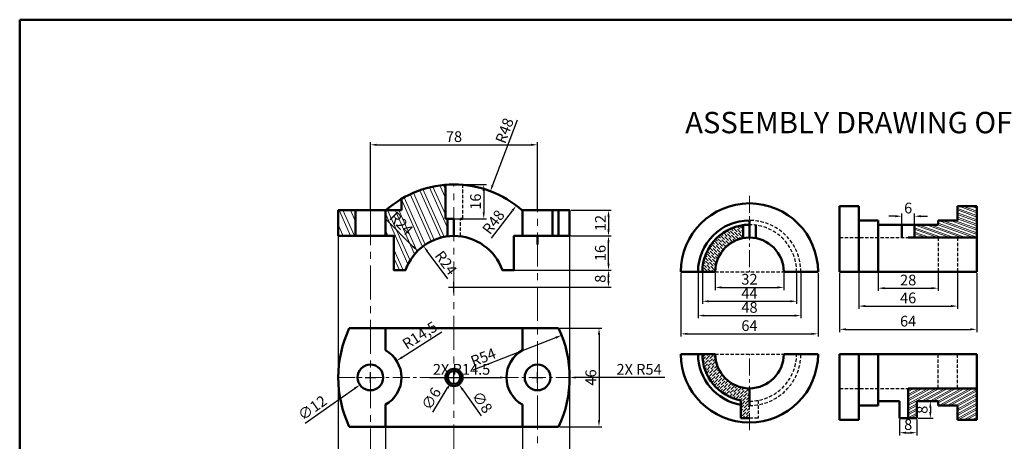
# Model space of a CAD drawing. Units: millimetres. Extents: x 6 to 817, y -61 to 407.
# Tile 2 of 3: x 6 to 466, y 210 to 407. Entities that reach past the tile are written whole.
import ezdxf

# ---------------------------------------------------------------- set-up
doc = ezdxf.new("R2010")
doc.units = ezdxf.units.MM
doc.header["$LTSCALE"] = 0.5
doc.linetypes.add('CENTER', pattern=[50.8, 31.75, -6.35, 6.35, -6.35])
doc.linetypes.add('HIDDEN', pattern=[9.525, 6.35, -3.175])
for name, color, linetype, lineweight in [('M-CNTR', 1, 'CENTER', 18), ('M-DIMS', 2, 'Continuous', 25), ('M-HATC', 8, 'Continuous', 18), ('M-HIDN', 4, 'HIDDEN', 25), ('M-OUTL', 7, 'Continuous', 50), ('M-TEXT', 3, 'Continuous', 25)]:
    doc.layers.add(name, color=color, linetype=linetype, lineweight=lineweight)
doc.styles.get("Standard").update_dxf_attribs({"font": 'arial.ttf'})
doc.dimstyles.new('ISO-25', dxfattribs={"dimtxt": 5, "dimasz": 3, "dimexe": 1.25, "dimexo": 0.625, "dimtad": 1, "dimtxsty": 'Standard', "dimcen": 2.5, "dimadec": 0, "dimazin": 0, "dimtfac": 1, "dimtofl": 0, "dimtmove": 0, "dimatfit": 3, "dimfxl": 1, "dimarcsym": 0})

# ---------------------------------------------------------------- blocks, each defined once
blk = doc.blocks.new('*D19')
at = {"layer": 'Defpoints', "color": 0, "ltscale": 0.5, "transparency": 16777216}
for p in [(257.89, 263.11), (257.89, 217.11), (276.73, 217.11)]:
    blk.add_point(p, dxfattribs=at)
at = {"layer": 'M-DIMS', "color": 0, "lineweight": -2, "ltscale": 0.5, "transparency": 16777216}
for p, q in [((258.51, 263.11), (277.98, 263.11)), ((276.73, 260.11), (276.73, 220.11)), ((258.51, 217.11), (277.98, 217.11))]:
    blk.add_line(p, q, dxfattribs=at)
at = {"layer": 'M-DIMS', "color": 0, "ltscale": 0.5, "transparency": 16777216}
for points in [[(276.23, 260.11), (277.23, 260.11), (276.73, 263.11)], [(276.23, 220.11), (277.23, 220.11), (276.73, 217.11)]]:
    blk.add_solid(points, dxfattribs=at)
at = {"layer": 'M-DIMS', "color": 0, "ltscale": 0.5, "transparency": 16777216, "insert": (273.55, 240.11), "char_height": 5, "attachment_point": 5, "rotation": 90}
blk.add_mtext('46', dxfattribs=at)
blk = doc.blocks.new('*D20')
at = {"layer": 'Defpoints', "color": 0, "ltscale": 0.5, "transparency": 16777216}
for p in [(182.27, 247.89), (170.03, 240.11)]:
    blk.add_point(p, dxfattribs=at)
at = {"layer": 'M-DIMS', "color": 0, "lineweight": -2, "ltscale": 0.5, "transparency": 16777216}
for p, q in [((203.42, 261.33), (184.8, 249.5)), ((167.53, 240.11), (172.53, 240.11)), ((170.03, 237.61), (170.03, 242.61))]:
    blk.add_line(p, q, dxfattribs=at)
at = {"layer": 'M-DIMS', "color": 0, "ltscale": 0.5, "transparency": 16777216}
blk.add_solid([(184.53, 249.92), (185.07, 249.08), (182.27, 247.89)], dxfattribs=at)
at = {"layer": 'M-DIMS', "color": 0, "ltscale": 0.5, "transparency": 16777216, "insert": (193.43, 259.28), "char_height": 5, "attachment_point": 5, "rotation": 32.4428}
blk.add_mtext('R14,5', dxfattribs=at)
blk = doc.blocks.new('*D21')
at = {"layer": 'Defpoints', "color": 0, "ltscale": 0.5, "transparency": 16777216}
for p in [(259.31, 259.81), (209.03, 240.11)]:
    blk.add_point(p, dxfattribs=at)
at = {"layer": 'M-DIMS', "color": 0, "lineweight": -2, "ltscale": 0.5, "transparency": 16777216}
blk.add_line((217.95, 243.6), (256.52, 258.72), dxfattribs=at)
at = {"layer": 'M-DIMS', "color": 0, "ltscale": 0.5, "transparency": 16777216}
blk.add_solid([(256.33, 259.18), (256.7, 258.25), (259.31, 259.81)], dxfattribs=at)
at = {"layer": 'M-DIMS', "color": 0, "ltscale": 0.5, "transparency": 16777216, "insert": (222.93, 248.96), "char_height": 5, "attachment_point": 5, "rotation": 21.398}
blk.add_mtext('R54', dxfattribs=at)
blk = doc.blocks.new('*D22')
at = {"layer": 'Defpoints', "color": 0, "ltscale": 0.5, "transparency": 16777216}
for p in [(174.94, 243.56), (165.12, 236.66)]:
    blk.add_point(p, dxfattribs=at)
at = {"layer": 'M-DIMS', "color": 0, "lineweight": -2, "ltscale": 0.5, "transparency": 16777216}
for p, q in [((167.53, 240.11), (172.53, 240.11)), ((170.03, 237.61), (170.03, 242.61)), ((139.54, 218.71), (162.66, 234.94))]:
    blk.add_line(p, q, dxfattribs=at)
at = {"layer": 'M-DIMS', "color": 0, "ltscale": 0.5, "transparency": 16777216}
blk.add_solid([(162.38, 235.35), (162.95, 234.53), (165.12, 236.66)], dxfattribs=at)
at = {"layer": 'M-DIMS', "color": 0, "ltscale": 0.5, "transparency": 16777216, "insert": (143.29, 225.39), "char_height": 5, "attachment_point": 5, "rotation": 35.0654}
blk.add_mtext('∅12', dxfattribs=at)
blk = doc.blocks.new('*D23')
at = {"layer": 'Defpoints', "color": 0, "ltscale": 0.5, "transparency": 16777216}
for p in [(206.69, 243.36), (211.37, 236.86)]:
    blk.add_point(p, dxfattribs=at)
at = {"layer": 'M-DIMS', "color": 0, "lineweight": -2, "ltscale": 0.5, "transparency": 16777216}
for p, q in [((206.53, 240.11), (211.53, 240.11)), ((209.03, 237.61), (209.03, 242.61)), ((221.92, 222.19), (213.12, 234.43))]:
    blk.add_line(p, q, dxfattribs=at)
at = {"layer": 'M-DIMS', "color": 0, "ltscale": 0.5, "transparency": 16777216}
blk.add_solid([(213.52, 234.72), (212.71, 234.14), (211.37, 236.86)], dxfattribs=at)
at = {"layer": 'M-DIMS', "color": 0, "ltscale": 0.5, "transparency": 16777216, "insert": (221.7, 228.18), "char_height": 5, "attachment_point": 5, "rotation": 305.7354}
blk.add_mtext('∅8', dxfattribs=at)
blk = doc.blocks.new('*D24')
at = {"layer": 'Defpoints', "color": 0, "ltscale": 0.5, "transparency": 16777216}
for p in [(210.58, 242.68), (207.48, 237.54)]:
    blk.add_point(p, dxfattribs=at)
at = {"layer": 'M-DIMS', "color": 0, "lineweight": -2, "ltscale": 0.5, "transparency": 16777216}
for p, q in [((206.53, 240.11), (211.53, 240.11)), ((209.03, 237.61), (209.03, 242.61)), ((199.24, 223.87), (205.93, 234.97))]:
    blk.add_line(p, q, dxfattribs=at)
at = {"layer": 'M-DIMS', "color": 0, "ltscale": 0.5, "transparency": 16777216}
blk.add_solid([(205.51, 235.23), (206.36, 234.71), (207.48, 237.54)], dxfattribs=at)
at = {"layer": 'M-DIMS', "color": 0, "ltscale": 0.5, "transparency": 16777216, "insert": (198.97, 229.85), "char_height": 5, "attachment_point": 5, "rotation": 58.929}
blk.add_mtext('∅6', dxfattribs=at)
blk = doc.blocks.new('*D25')
at = {"layer": 'Defpoints', "color": 0, "ltscale": 0.5, "transparency": 16777216}
for p in [(263.03, 318.23), (263.03, 306.23), (281.16, 306.23)]:
    blk.add_point(p, dxfattribs=at)
at = {"layer": 'M-DIMS', "color": 0, "lineweight": -2, "ltscale": 0.5, "transparency": 16777216}
for p, q in [((263.66, 318.23), (282.41, 318.23)), ((281.16, 315.23), (281.16, 309.23)), ((263.66, 306.23), (282.41, 306.23))]:
    blk.add_line(p, q, dxfattribs=at)
at = {"layer": 'M-DIMS', "color": 0, "ltscale": 0.5, "transparency": 16777216}
for points in [[(280.66, 315.23), (281.66, 315.23), (281.16, 318.23)], [(280.66, 309.23), (281.66, 309.23), (281.16, 306.23)]]:
    blk.add_solid(points, dxfattribs=at)
at = {"layer": 'M-DIMS', "color": 0, "ltscale": 0.5, "transparency": 16777216, "insert": (278.02, 312.23), "char_height": 5, "attachment_point": 5, "rotation": 90}
blk.add_mtext('12', dxfattribs=at)
blk = doc.blocks.new('*D26')
at = {"layer": 'Defpoints', "color": 0, "ltscale": 0.5, "transparency": 16777216}
for p in [(237.03, 306.23), (281.16, 306.23), (237.03, 290.23)]:
    blk.add_point(p, dxfattribs=at)
at = {"layer": 'M-DIMS', "color": 0, "lineweight": -2, "ltscale": 0.5, "transparency": 16777216}
for p, q in [((237.66, 306.23), (282.41, 306.23)), ((281.16, 293.23), (281.16, 303.23)), ((237.66, 290.23), (282.41, 290.23))]:
    blk.add_line(p, q, dxfattribs=at)
at = {"layer": 'M-DIMS', "color": 0, "ltscale": 0.5, "transparency": 16777216}
for points in [[(280.66, 303.23), (281.66, 303.23), (281.16, 306.23)], [(280.66, 293.23), (281.66, 293.23), (281.16, 290.23)]]:
    blk.add_solid(points, dxfattribs=at)
at = {"layer": 'M-DIMS', "color": 0, "ltscale": 0.5, "transparency": 16777216, "insert": (277.98, 298.23), "char_height": 5, "attachment_point": 5, "rotation": 90}
blk.add_mtext('16', dxfattribs=at)
blk = doc.blocks.new('*D27')
at = {"layer": 'Defpoints', "color": 0, "ltscale": 0.5, "transparency": 16777216}
for p in [(231.66, 290.23), (281.16, 290.23), (209.03, 282.23)]:
    blk.add_point(p, dxfattribs=at)
at = {"layer": 'M-DIMS', "color": 0, "lineweight": -2, "ltscale": 0.5, "transparency": 16777216}
for p, q in [((232.28, 290.23), (282.41, 290.23)), ((281.16, 285.23), (281.16, 287.23)), ((209.66, 282.23), (282.41, 282.23))]:
    blk.add_line(p, q, dxfattribs=at)
at = {"layer": 'M-DIMS', "color": 0, "ltscale": 0.5, "transparency": 16777216}
for points in [[(280.66, 287.23), (281.66, 287.23), (281.16, 290.23)], [(280.66, 285.23), (281.66, 285.23), (281.16, 282.23)]]:
    blk.add_solid(points, dxfattribs=at)
at = {"layer": 'M-DIMS', "color": 0, "ltscale": 0.5, "transparency": 16777216, "insert": (277.98, 286.23), "char_height": 5, "attachment_point": 5, "rotation": 90}
blk.add_mtext('8', dxfattribs=at)
blk = doc.blocks.new('*D28')
at = {"layer": 'Defpoints', "color": 0, "ltscale": 0.5, "transparency": 16777216}
for p in [(209.03, 330.23), (209.03, 314.23), (222.93, 314.23)]:
    blk.add_point(p, dxfattribs=at)
at = {"layer": 'M-DIMS', "color": 0, "lineweight": -2, "ltscale": 0.5, "transparency": 16777216}
for p, q in [((209.66, 330.23), (224.18, 330.23)), ((222.93, 327.23), (222.93, 317.23)), ((209.66, 314.23), (224.18, 314.23))]:
    blk.add_line(p, q, dxfattribs=at)
at = {"layer": 'M-DIMS', "color": 0, "ltscale": 0.5, "transparency": 16777216}
for points in [[(222.43, 327.23), (223.43, 327.23), (222.93, 330.23)], [(222.43, 317.23), (223.43, 317.23), (222.93, 314.23)]]:
    blk.add_solid(points, dxfattribs=at)
at = {"layer": 'M-DIMS', "color": 0, "ltscale": 0.5, "transparency": 16777216, "insert": (219.75, 322.23), "char_height": 5, "attachment_point": 5, "rotation": 90}
blk.add_mtext('16', dxfattribs=at)
blk = doc.blocks.new('*D29')
at = {"layer": 'Defpoints', "color": 0, "ltscale": 0.5, "transparency": 16777216}
for p in [(194.8, 301.55), (209.03, 282.23)]:
    blk.add_point(p, dxfattribs=at)
at = {"layer": 'M-DIMS', "color": 0, "lineweight": -2, "ltscale": 0.5, "transparency": 16777216}
blk.add_line((206.17, 286.11), (196.58, 299.14), dxfattribs=at)
at = {"layer": 'M-DIMS', "color": 0, "ltscale": 0.5, "transparency": 16777216}
blk.add_solid([(196.98, 299.43), (196.18, 298.84), (194.8, 301.55)], dxfattribs=at)
at = {"layer": 'M-DIMS', "color": 0, "ltscale": 0.5, "transparency": 16777216, "insert": (204.79, 293.28), "char_height": 5, "attachment_point": 5, "rotation": 306.3657}
blk.add_mtext('R24', dxfattribs=at)
blk = doc.blocks.new('*D30')
at = {"layer": 'Defpoints', "color": 0, "ltscale": 0.5, "transparency": 16777216}
for p in [(238.13, 320.4), (209.03, 282.23)]:
    blk.add_point(p, dxfattribs=at)
at = {"layer": 'M-DIMS', "color": 0, "lineweight": -2, "ltscale": 0.5, "transparency": 16777216}
blk.add_line((226.48, 305.13), (236.31, 318.02), dxfattribs=at)
at = {"layer": 'M-DIMS', "color": 0, "ltscale": 0.5, "transparency": 16777216}
blk.add_solid([(235.91, 318.32), (236.71, 317.71), (238.13, 320.4)], dxfattribs=at)
at = {"layer": 'M-DIMS', "color": 0, "ltscale": 0.5, "transparency": 16777216, "insert": (227.96, 312.31), "char_height": 5, "attachment_point": 5, "rotation": 52.6886}
blk.add_mtext('R48', dxfattribs=at)
blk = doc.blocks.new('*D31')
at = {"layer": 'Defpoints', "color": 0, "ltscale": 0.5, "transparency": 16777216}
for p in [(330.95, 289.45), (362.95, 289.45), (362.95, 282.17)]:
    blk.add_point(p, dxfattribs=at)
at = {"layer": 'M-DIMS', "color": 0, "lineweight": -2, "ltscale": 0.5, "transparency": 16777216}
for p, q in [((330.95, 288.83), (330.95, 280.92)), ((362.95, 288.83), (362.95, 280.92)), ((333.95, 282.17), (359.95, 282.17))]:
    blk.add_line(p, q, dxfattribs=at)
at = {"layer": 'M-DIMS', "color": 0, "ltscale": 0.5, "transparency": 16777216}
for points in [[(333.95, 282.67), (333.95, 281.67), (330.95, 282.17)], [(359.95, 282.67), (359.95, 281.67), (362.95, 282.17)]]:
    blk.add_solid(points, dxfattribs=at)
at = {"layer": 'M-DIMS', "color": 0, "ltscale": 0.5, "transparency": 16777216, "insert": (346.95, 285.35), "char_height": 5, "attachment_point": 5}
blk.add_mtext('32', dxfattribs=at)
blk = doc.blocks.new('*D32')
at = {"layer": 'Defpoints', "color": 0, "ltscale": 0.5, "transparency": 16777216}
for p in [(324.95, 289.45), (368.95, 289.45), (368.95, 275.69)]:
    blk.add_point(p, dxfattribs=at)
at = {"layer": 'M-DIMS', "color": 0, "lineweight": -2, "ltscale": 0.5, "transparency": 16777216}
for p, q in [((324.95, 288.83), (324.95, 274.44)), ((368.95, 288.83), (368.95, 274.44)), ((327.95, 275.69), (365.95, 275.69))]:
    blk.add_line(p, q, dxfattribs=at)
at = {"layer": 'M-DIMS', "color": 0, "ltscale": 0.5, "transparency": 16777216}
for points in [[(327.95, 276.19), (327.95, 275.19), (324.95, 275.69)], [(365.95, 276.19), (365.95, 275.19), (368.95, 275.69)]]:
    blk.add_solid(points, dxfattribs=at)
at = {"layer": 'M-DIMS', "color": 0, "ltscale": 0.5, "transparency": 16777216, "insert": (346.95, 278.81), "char_height": 5, "attachment_point": 5}
blk.add_mtext('44', dxfattribs=at)
blk = doc.blocks.new('*D33')
at = {"layer": 'Defpoints', "color": 0, "ltscale": 0.5, "transparency": 16777216}
for p in [(322.95, 289.45), (370.95, 289.45), (370.95, 269.02)]:
    blk.add_point(p, dxfattribs=at)
at = {"layer": 'M-DIMS', "color": 0, "lineweight": -2, "ltscale": 0.5, "transparency": 16777216}
for p, q in [((322.95, 288.83), (322.95, 267.77)), ((370.95, 288.83), (370.95, 267.77)), ((325.95, 269.02), (367.95, 269.02))]:
    blk.add_line(p, q, dxfattribs=at)
at = {"layer": 'M-DIMS', "color": 0, "ltscale": 0.5, "transparency": 16777216}
for points in [[(325.95, 269.52), (325.95, 268.52), (322.95, 269.02)], [(367.95, 269.52), (367.95, 268.52), (370.95, 269.02)]]:
    blk.add_solid(points, dxfattribs=at)
at = {"layer": 'M-DIMS', "color": 0, "ltscale": 0.5, "transparency": 16777216, "insert": (346.95, 272.19), "char_height": 5, "attachment_point": 5}
blk.add_mtext('48', dxfattribs=at)
blk = doc.blocks.new('*D34')
at = {"layer": 'Defpoints', "color": 0, "ltscale": 0.5, "transparency": 16777216}
for p in [(314.95, 289.45), (378.95, 289.45), (378.95, 260.49)]:
    blk.add_point(p, dxfattribs=at)
at = {"layer": 'M-DIMS', "color": 0, "lineweight": -2, "ltscale": 0.5, "transparency": 16777216}
for p, q in [((314.95, 288.83), (314.95, 259.24)), ((378.95, 288.83), (378.95, 259.24)), ((317.95, 260.49), (375.95, 260.49))]:
    blk.add_line(p, q, dxfattribs=at)
at = {"layer": 'M-DIMS', "color": 0, "ltscale": 0.5, "transparency": 16777216}
for points in [[(317.95, 260.99), (317.95, 259.99), (314.95, 260.49)], [(375.95, 260.99), (375.95, 259.99), (378.95, 260.49)]]:
    blk.add_solid(points, dxfattribs=at)
at = {"layer": 'M-DIMS', "color": 0, "ltscale": 0.5, "transparency": 16777216, "insert": (346.95, 263.67), "char_height": 5, "attachment_point": 5}
blk.add_mtext('64', dxfattribs=at)
blk = doc.blocks.new('*D35')
at = {"layer": 'Defpoints', "color": 0, "ltscale": 0.5, "transparency": 16777216}
for p in [(417.01, 221.03), (425.01, 221.03), (425.01, 214.3)]:
    blk.add_point(p, dxfattribs=at)
at = {"layer": 'M-DIMS', "color": 0, "lineweight": -2, "ltscale": 0.5, "transparency": 16777216}
for p, q in [((417.01, 220.41), (417.01, 213.05)), ((425.01, 220.41), (425.01, 213.05)), ((420.01, 214.3), (422.01, 214.3))]:
    blk.add_line(p, q, dxfattribs=at)
at = {"layer": 'M-DIMS', "color": 0, "ltscale": 0.5, "transparency": 16777216}
for points in [[(420.01, 214.8), (420.01, 213.8), (417.01, 214.3)], [(422.01, 214.8), (422.01, 213.8), (425.01, 214.3)]]:
    blk.add_solid(points, dxfattribs=at)
at = {"layer": 'M-DIMS', "color": 0, "ltscale": 0.5, "transparency": 16777216, "insert": (421.01, 217.48), "char_height": 5, "attachment_point": 5}
blk.add_mtext('8', dxfattribs=at)
blk = doc.blocks.new('*D36')
at = {"layer": 'Defpoints', "color": 0, "ltscale": 0.5, "transparency": 16777216}
for p in [(425.03, 229.03), (425.03, 221.03), (431.36, 221.03)]:
    blk.add_point(p, dxfattribs=at)
at = {"layer": 'M-DIMS', "color": 0, "lineweight": -2, "ltscale": 0.5, "transparency": 16777216}
for p, q in [((425.65, 229.03), (432.61, 229.03)), ((431.36, 226.03), (431.36, 224.03)), ((425.65, 221.03), (432.61, 221.03))]:
    blk.add_line(p, q, dxfattribs=at)
at = {"layer": 'M-DIMS', "color": 0, "ltscale": 0.5, "transparency": 16777216}
for points in [[(430.86, 226.03), (431.86, 226.03), (431.36, 229.03)], [(430.86, 224.03), (431.86, 224.03), (431.36, 221.03)]]:
    blk.add_solid(points, dxfattribs=at)
at = {"layer": 'M-DIMS', "color": 0, "ltscale": 0.5, "transparency": 16777216, "insert": (428.18, 225.03), "char_height": 5, "attachment_point": 5, "rotation": 90}
blk.add_mtext('8', dxfattribs=at)
blk = doc.blocks.new('*D37')
at = {"layer": 'Defpoints', "color": 0, "ltscale": 0.5, "transparency": 16777216}
for p in [(407.01, 289.45), (435.01, 289.45), (435.01, 281.8)]:
    blk.add_point(p, dxfattribs=at)
at = {"layer": 'M-DIMS', "color": 0, "lineweight": -2, "ltscale": 0.5, "transparency": 16777216}
for p, q in [((407.01, 288.83), (407.01, 280.55)), ((435.01, 288.83), (435.01, 280.55)), ((410.01, 281.8), (432.01, 281.8))]:
    blk.add_line(p, q, dxfattribs=at)
at = {"layer": 'M-DIMS', "color": 0, "ltscale": 0.5, "transparency": 16777216}
for points in [[(410.01, 282.3), (410.01, 281.3), (407.01, 281.8)], [(432.01, 282.3), (432.01, 281.3), (435.01, 281.8)]]:
    blk.add_solid(points, dxfattribs=at)
at = {"layer": 'M-DIMS', "color": 0, "ltscale": 0.5, "transparency": 16777216, "insert": (421.01, 284.98), "char_height": 5, "attachment_point": 5}
blk.add_mtext('28', dxfattribs=at)
blk = doc.blocks.new('*D38')
at = {"layer": 'Defpoints', "color": 0, "ltscale": 0.5, "transparency": 16777216}
for p in [(398.01, 289.45), (444.01, 289.45), (444.01, 273.46)]:
    blk.add_point(p, dxfattribs=at)
at = {"layer": 'M-DIMS', "color": 0, "lineweight": -2, "ltscale": 0.5, "transparency": 16777216}
for p, q in [((398.01, 288.83), (398.01, 272.21)), ((444.01, 288.83), (444.01, 272.21)), ((401.01, 273.46), (441.01, 273.46))]:
    blk.add_line(p, q, dxfattribs=at)
at = {"layer": 'M-DIMS', "color": 0, "ltscale": 0.5, "transparency": 16777216}
for points in [[(401.01, 273.96), (401.01, 272.96), (398.01, 273.46)], [(441.01, 273.96), (441.01, 272.96), (444.01, 273.46)]]:
    blk.add_solid(points, dxfattribs=at)
at = {"layer": 'M-DIMS', "color": 0, "ltscale": 0.5, "transparency": 16777216, "insert": (421.01, 276.64), "char_height": 5, "attachment_point": 5}
blk.add_mtext('46', dxfattribs=at)
blk = doc.blocks.new('*D39')
at = {"layer": 'Defpoints', "color": 0, "ltscale": 0.5, "transparency": 16777216}
for p in [(389.01, 289.45), (453.01, 289.45), (453.01, 262.59)]:
    blk.add_point(p, dxfattribs=at)
at = {"layer": 'M-DIMS', "color": 0, "lineweight": -2, "ltscale": 0.5, "transparency": 16777216}
for p, q in [((389.01, 288.83), (389.01, 261.34)), ((453.01, 288.83), (453.01, 261.34)), ((392.01, 262.59), (450.01, 262.59))]:
    blk.add_line(p, q, dxfattribs=at)
at = {"layer": 'M-DIMS', "color": 0, "ltscale": 0.5, "transparency": 16777216}
for points in [[(392.01, 263.09), (392.01, 262.09), (389.01, 262.59)], [(450.01, 263.09), (450.01, 262.09), (453.01, 262.59)]]:
    blk.add_solid(points, dxfattribs=at)
at = {"layer": 'M-DIMS', "color": 0, "ltscale": 0.5, "transparency": 16777216, "insert": (421.01, 265.77), "char_height": 5, "attachment_point": 5}
blk.add_mtext('64', dxfattribs=at)
blk = doc.blocks.new('*D40')
at = {"layer": 'Defpoints', "color": 0, "ltscale": 0.5, "transparency": 16777216}
for p in [(424.01, 315.42), (418.01, 311.45), (424.01, 311.45)]:
    blk.add_point(p, dxfattribs=at)
at = {"layer": 'M-DIMS', "color": 0, "lineweight": -2, "ltscale": 0.5, "transparency": 16777216}
for p, q in [((415.01, 315.42), (412.01, 315.42)), ((418.01, 312.08), (418.01, 316.67)), ((424.01, 312.08), (424.01, 316.67)), ((427.01, 315.42), (430.01, 315.42))]:
    blk.add_line(p, q, dxfattribs=at)
at = {"layer": 'M-DIMS', "color": 0, "ltscale": 0.5, "transparency": 16777216}
for points in [[(415.01, 315.92), (415.01, 314.92), (418.01, 315.42)], [(427.01, 315.92), (427.01, 314.92), (424.01, 315.42)]]:
    blk.add_solid(points, dxfattribs=at)
at = {"layer": 'M-DIMS', "color": 0, "ltscale": 0.5, "transparency": 16777216, "insert": (421.01, 318.6), "char_height": 5, "attachment_point": 5}
blk.add_mtext('6', dxfattribs=at)
blk = doc.blocks.new('*D51')
at = {"layer": 'Defpoints', "color": 0, "ltscale": 0.5, "transparency": 16777216}
for p in [(155.03, 306.23), (263.03, 306.23), (263.03, 5.88)]:
    blk.add_point(p, dxfattribs=at)
at = {"layer": 'M-DIMS', "color": 0, "lineweight": -2, "ltscale": 0.5, "transparency": 16777216}
for p, q in [((155.03, 305.6), (155.03, 4.63)), ((263.03, 305.6), (263.03, 4.63)), ((158.03, 5.88), (260.03, 5.88))]:
    blk.add_line(p, q, dxfattribs=at)
at = {"layer": 'M-DIMS', "color": 0, "ltscale": 0.5, "transparency": 16777216}
for points in [[(158.03, 6.38), (158.03, 5.38), (155.03, 5.88)], [(260.03, 6.38), (260.03, 5.38), (263.03, 5.88)]]:
    blk.add_solid(points, dxfattribs=at)
at = {"layer": 'M-DIMS', "color": 0, "ltscale": 0.5, "transparency": 16777216, "insert": (209.03, 9.06), "char_height": 5, "attachment_point": 5}
blk.add_mtext('108', dxfattribs=at)
blk = doc.blocks.new('*D52')
at = {"layer": 'Defpoints', "color": 0, "ltscale": 0.5, "transparency": 16777216}
for p in [(248.03, 348.78), (170.03, 318.23), (248.03, 318.23)]:
    blk.add_point(p, dxfattribs=at)
at = {"layer": 'M-DIMS', "color": 0, "lineweight": -2, "ltscale": 0.5, "transparency": 16777216}
for p, q in [((170.03, 318.85), (170.03, 350.03)), ((248.03, 318.85), (248.03, 350.03)), ((173.03, 348.78), (245.03, 348.78))]:
    blk.add_line(p, q, dxfattribs=at)
at = {"layer": 'M-DIMS', "color": 0, "ltscale": 0.5, "transparency": 16777216}
for points in [[(173.03, 349.28), (173.03, 348.28), (170.03, 348.78)], [(245.03, 349.28), (245.03, 348.28), (248.03, 348.78)]]:
    blk.add_solid(points, dxfattribs=at)
at = {"layer": 'M-DIMS', "color": 0, "ltscale": 0.5, "transparency": 16777216, "insert": (209.03, 351.96), "char_height": 5, "attachment_point": 5}
blk.add_mtext('78', dxfattribs=at)
blk = doc.blocks.new('*D53')
at = {"layer": 'Defpoints', "color": 0, "ltscale": 0.5, "transparency": 16777216}
for p in [(177.03, 217.11), (241.03, 217.11), (241.03, 5.88)]:
    blk.add_point(p, dxfattribs=at)
at = {"layer": 'M-DIMS', "color": 0, "lineweight": -2, "ltscale": 0.5, "transparency": 16777216}
for p, q in [((177.03, 216.48), (177.03, 4.63)), ((241.03, 216.48), (241.03, 4.63)), ((180.03, 5.88), (238.03, 5.88))]:
    blk.add_line(p, q, dxfattribs=at)
at = {"layer": 'M-DIMS', "color": 0, "ltscale": 0.5, "transparency": 16777216}
for points in [[(180.03, 6.38), (180.03, 5.38), (177.03, 5.88)], [(238.03, 6.38), (238.03, 5.38), (241.03, 5.88)]]:
    blk.add_solid(points, dxfattribs=at)
at = {"layer": 'M-DIMS', "color": 0, "ltscale": 0.5, "transparency": 16777216, "insert": (209.03, 9.06), "char_height": 5, "attachment_point": 5}
blk.add_mtext('64', dxfattribs=at)
blk = doc.blocks.new('*D57')
at = {"layer": 'Defpoints', "color": 0, "ltscale": 0.5, "transparency": 16777216}
for p in [(226.01, 327.12), (209.03, 282.23)]:
    blk.add_point(p, dxfattribs=at)
at = {"layer": 'M-DIMS', "color": 0, "lineweight": -2, "ltscale": 0.5, "transparency": 16777216}
for p, q in [((238.53, 360.24), (227.07, 329.93)), ((206.53, 282.23), (211.53, 282.23)), ((209.03, 279.73), (209.03, 284.73))]:
    blk.add_line(p, q, dxfattribs=at)
at = {"layer": 'M-DIMS', "color": 0, "ltscale": 0.5, "transparency": 16777216}
blk.add_solid([(226.6, 330.11), (227.54, 329.75), (226.01, 327.12)], dxfattribs=at)
at = {"layer": 'M-DIMS', "color": 0, "ltscale": 0.5, "transparency": 16777216, "insert": (233.22, 355.19), "char_height": 5, "attachment_point": 5, "rotation": 69.2852}
blk.add_mtext('R48', dxfattribs=at)
blk = doc.blocks.new('*D58')
at = {"layer": 'Defpoints', "color": 0, "ltscale": 0.5, "transparency": 16777216}
for p in [(192.03, 299.17), (209.03, 282.23)]:
    blk.add_point(p, dxfattribs=at)
at = {"layer": 'M-DIMS', "color": 0, "lineweight": -2, "ltscale": 0.5, "transparency": 16777216}
for p, q in [((177.16, 313.98), (189.91, 301.29)), ((206.53, 282.23), (211.53, 282.23)), ((209.03, 279.73), (209.03, 284.73))]:
    blk.add_line(p, q, dxfattribs=at)
at = {"layer": 'M-DIMS', "color": 0, "ltscale": 0.5, "transparency": 16777216}
blk.add_solid([(190.26, 301.64), (189.55, 300.93), (192.03, 299.17)], dxfattribs=at)
at = {"layer": 'M-DIMS', "color": 0, "ltscale": 0.5, "transparency": 16777216, "insert": (184.04, 311.55), "char_height": 5, "attachment_point": 5, "rotation": 315.0976}
blk.add_mtext('R24', dxfattribs=at)
blk = doc.blocks.new('*D59')
at = {"layer": 'Defpoints', "color": 0, "ltscale": 0.5, "transparency": 16777216}
for p in [(233.53, 240.1), (248.03, 240.11)]:
    blk.add_point(p, dxfattribs=at)
at = {"layer": 'M-DIMS', "color": 0, "lineweight": -2, "ltscale": 0.5, "transparency": 16777216}
for p, q in [((197.64, 240.08), (230.53, 240.1)), ((245.53, 240.11), (250.53, 240.11)), ((248.03, 237.61), (248.03, 242.61))]:
    blk.add_line(p, q, dxfattribs=at)
at = {"layer": 'M-DIMS', "color": 0, "ltscale": 0.5, "transparency": 16777216}
blk.add_solid([(230.53, 240.6), (230.53, 239.6), (233.53, 240.1)], dxfattribs=at)
at = {"layer": 'M-DIMS', "color": 0, "ltscale": 0.5, "transparency": 16777216, "insert": (212.58, 243.26), "char_height": 5, "attachment_point": 5, "rotation": 0.0366}
blk.add_mtext('2X R14.5', dxfattribs=at)
blk = doc.blocks.new('*D60')
at = {"layer": 'Defpoints', "color": 0, "ltscale": 0.5, "transparency": 16777216}
for p in [(209.03, 240.11), (263.03, 240.1)]:
    blk.add_point(p, dxfattribs=at)
at = {"layer": 'M-DIMS', "color": 0, "lineweight": -2, "ltscale": 0.5, "transparency": 16777216}
for p, q in [((206.53, 240.11), (211.53, 240.11)), ((209.03, 237.61), (209.03, 242.61)), ((307.43, 240.09), (266.03, 240.1))]:
    blk.add_line(p, q, dxfattribs=at)
at = {"layer": 'M-DIMS', "color": 0, "ltscale": 0.5, "transparency": 16777216}
blk.add_solid([(266.03, 240.6), (266.03, 239.6), (263.03, 240.1)], dxfattribs=at)
at = {"layer": 'M-DIMS', "color": 0, "ltscale": 0.5, "transparency": 16777216, "insert": (295.43, 243.27), "char_height": 5, "attachment_point": 5, "rotation": 359.9901}
blk.add_mtext('2X R54', dxfattribs=at)

msp = doc.modelspace()

# ---------------------------------------------------------------- hatches: boundary and pattern name
at = {"layer": 'M-HATC', "ltscale": 0.5}
h = msp.add_hatch(dxfattribs=at)
h.set_pattern_fill('ANSI32', color=256, scale=0.5, angle=69)
h.paths.add_polyline_path([(206.031, 314.227), (205.031, 314.227), (205.031, 330.06, 0.113544), (184.531, 323.504), (184.531, 318.227), (177.282, 318.227), (177.031, 318.227), (177.031, 306.227), (181.031, 306.227), (181.031, 302.227), (181.031, 290.227), (186.403, 290.227, -0.2836692), (206.031, 306.039)])
h.paths.add_polyline_path([(163.031, 318.227), (155.031, 318.227), (155.031, 306.227), (163.031, 306.227)])
h = msp.add_hatch(dxfattribs=at)
h.set_pattern_fill('ANSI32', color=256, scale=0.2, angle=115)
h.set_pattern_definition([(160, (-84.5117, -12.3327), (-0.6515484, -1.7901144), []), (160, (-84.8912, -11.5188), (-0.6515484, -1.7901144), [])])
h.paths.add_polyline_path([(453.012, 305.451), (453.012, 320.152), (444.012, 320.152), (444.012, 313.451), (435.012, 313.451), (435.012, 311.451), (424.012, 311.451), (424.012, 305.451)])
h = msp.add_hatch(dxfattribs=at)
h.set_pattern_fill('ANSI36', color=256, scale=0.3, angle=90)
h.paths.add_polyline_path([(343.952, 311.246, 0.3746932), (324.952, 289.451), (330.952, 289.451, -0.359988), (343.952, 305.168)])
h = msp.add_hatch(dxfattribs=at)
h.set_pattern_fill('ANSI36', color=256, scale=0.3)
h.paths.add_polyline_path([(330.952, 251.033), (324.952, 251.033, 0.3616215), (342.952, 229.4), (342.952, 221.033), (346.952, 221.033), (346.952, 235.033, -0.4142136)])
h = msp.add_hatch(dxfattribs=at)
h.set_pattern_fill('ANSI32', color=256, scale=0.2, angle=164)
h.set_pattern_definition([(209, (-84.5117, -22.6975), (0.9235623, -1.6661505), []), (209, (-85.375, -22.45), (0.9235623, -1.6661505), [])])
h.paths.add_polyline_path([(444.012, 227.033), (444.012, 220.332), (453.012, 220.332), (453.012, 235.033), (421.012, 235.033), (421.012, 221.033), (425.012, 221.033), (425.012, 229.033), (435.012, 229.033), (435.012, 227.033)])

# ---------------------------------------------------------------- linework, layer by layer
at = {"layer": 'M-CNTR'}
for p, q in [((209.031, 24.431), (209.031, 330.227)), ((170.031, 124.143), (170.031, 318.227)), ((248.031, 114.143), (248.031, 318.227))]:
    msp.add_line(p, q, dxfattribs=at)
at = {"layer": 'M-CNTR', "ltscale": 0.5}
for p, q in [((346.952, 324.926), (346.952, 289.451)), ((346.952, 215.559), (346.952, 251.033)), ((155.031, 240.109), (263.031, 240.109))]:
    msp.add_line(p, q, dxfattribs=at)
at = {"layer": 'M-HIDN', "ltscale": 0.5}
for p, q in [((213.031, 330.227), (213.031, 314.227)), ((209.031, 314.227), (212.031, 314.227)), ((212.031, 306.227), (212.031, 314.227)), ((389.012, 305.451), (421.012, 305.451)), ((435.012, 305.451), (435.012, 289.451)), ((444.012, 305.451), (444.012, 289.451)), ((330.952, 289.451), (362.952, 289.451)), ((330.952, 251.033), (362.952, 251.033)), ((435.012, 235.033), (435.012, 251.033)), ((444.012, 235.033), (444.012, 251.033)), ((389.012, 235.033), (421.012, 235.033)), ((350.952, 229.4), (350.952, 221.033)), ((350.952, 221.033), (346.952, 221.033))]:
    msp.add_line(p, q, dxfattribs=at)
for centre, radius, start, end in [((346.952, 289.451), 24, 0, 90), ((346.952, 289.451), 22, 0, 90), ((346.952, 251.033), 22, 270, 0), ((346.952, 251.033), 24, 270, 0)]:
    msp.add_arc(centre, radius, start, end, dxfattribs=at)
at = {"layer": 'M-OUTL', "ltscale": 0.5}
for p, q in [((205.031, 330.227), (205.031, 314.227)), ((184.531, 318.227), (184.531, 323.504)), ((163.031, 318.227), (163.031, 306.227)), ((177.031, 318.227), (177.031, 306.227)), ((177.282, 318.227), (184.531, 318.227)), ((241.031, 306.227), (241.031, 318.227)), ((255.031, 306.227), (255.031, 318.227)), ((257.888, 306.227), (257.888, 318.227)), ((263.031, 306.227), (263.031, 318.227)), ((389.012, 320.152), (389.012, 289.451)), ((389.012, 320.152), (398.012, 320.152)), ((398.012, 320.152), (398.012, 289.451)), ((444.012, 320.152), (444.012, 313.451)), ((444.012, 320.152), (453.012, 320.152)), ((453.012, 320.152), (453.012, 289.451)), ((205.031, 314.227), (209.031, 314.227)), ((206.031, 306.039), (206.031, 314.227)), ((209.031, 306.227), (209.031, 314.227)), ((212.031, 314.227), (213.031, 314.227)), ((346.952, 311.451), (346.952, 313.451)), ((346.952, 313.451), (346.952, 305.451)), ((398.012, 313.451), (407.012, 313.451)), ((407.012, 313.451), (407.012, 289.451)), ((435.012, 313.451), (435.012, 311.451)), ((435.012, 313.451), (444.012, 313.451)), ((343.952, 311.246), (343.952, 305.168)), ((349.952, 311.246), (349.952, 305.168)), ((407.012, 311.451), (435.012, 311.451)), ((418.012, 311.451), (418.012, 305.451)), ((424.012, 311.451), (424.012, 305.451)), ((248.031, 302.227), (248.031, 306.227)), ((421.012, 305.451), (453.012, 305.451)), ((314.952, 289.451), (330.952, 289.451)), ((362.952, 289.451), (378.952, 289.451)), ((389.012, 289.451), (453.012, 289.451)), ((160.174, 263.109), (257.888, 263.109)), ((177.031, 252.808), (177.031, 263.109)), ((241.031, 252.808), (241.031, 263.109)), ((314.952, 251.033), (330.952, 251.033)), ((362.952, 251.033), (378.952, 251.033)), ((389.012, 220.332), (389.012, 251.033)), ((389.012, 251.033), (453.012, 251.033)), ((398.012, 220.332), (398.012, 251.033)), ((407.012, 227.033), (407.012, 251.033)), ((453.012, 220.332), (453.012, 251.033)), ((346.952, 227.033), (346.952, 235.033)), ((421.012, 235.033), (453.012, 235.033)), ((421.012, 221.033), (421.012, 235.033)), ((177.031, 217.109), (177.031, 227.411)), ((241.031, 217.109), (241.031, 227.411)), ((342.952, 229.4), (342.952, 221.033)), ((398.012, 227.033), (407.012, 227.033)), ((407.012, 229.033), (417.012, 229.033)), ((417.012, 221.033), (417.012, 229.033)), ((425.012, 229.033), (425.012, 221.033)), ((425.012, 229.033), (435.012, 229.033)), ((435.012, 227.033), (435.012, 229.033)), ((435.012, 227.033), (444.012, 227.033)), ((444.012, 220.332), (444.012, 227.033)), ((346.952, 221.033), (342.952, 221.033)), ((425.012, 221.033), (417.012, 221.033)), ((160.174, 217.109), (257.888, 217.109)), ((389.012, 220.332), (398.012, 220.332)), ((444.012, 220.332), (453.012, 220.332))]:
    msp.add_line(p, q, dxfattribs=at)
msp.add_lwpolyline([(6.354, 407.228), (817.271, 407.228), (817.271, -60.955), (6.354, -60.955)], close=True, dxfattribs=at)
for points in [[(209.031, 330.227, 0.1826758), (177.282, 318.227), (155.031, 318.227), (155.031, 306.227), (181.031, 306.227), (181.031, 302.227), (181.031, 290.227), (186.403, 290.227, -0.3178372), (209.031, 306.227)], [(209.031, 330.227, -0.1826758), (240.78, 318.227), (263.031, 318.227), (263.031, 306.227), (237.031, 306.227), (237.031, 302.227), (237.031, 290.227), (231.658, 290.227, 0.3178372), (209.031, 306.227)]]:
    msp.add_lwpolyline(points, format="xyb", dxfattribs=at)
for centre, radius in [((170.031, 240.109), 6), ((209.031, 240.109), 4), ((248.031, 240.109), 6), ((209.031, 240.109), 3)]:
    msp.add_circle(centre, radius, dxfattribs=at)
for centre, radius, start, end in [((346.952, 289.451), 32, 0, 180), ((346.952, 289.451), 24, 90, 180), ((346.952, 289.451), 22, 90, 180), ((346.952, 289.451), 16, 0, 180), ((209.031, 240.109), 54, 154.79071, 205.20929), ((209.031, 240.109), 54, 334.79071, 25.20929), ((170.031, 240.109), 14.5, 298.86573, 61.13427), ((248.031, 240.109), 14.5, 118.86573, 241.13427), ((346.952, 251.033), 32, 180, 0), ((346.952, 251.033), 24, 180, 260.40593), ((346.952, 251.033), 22, 180, 259.52432), ((346.952, 251.033), 16, 180, 0)]:
    msp.add_arc(centre, radius, start, end, dxfattribs=at)

# ---------------------------------------------------------------- texts
at = {"layer": 'M-TEXT', "ltscale": 0.5, "insert": (316.953, 364.17), "char_height": 10, "attachment_point": 1}
msp.add_mtext_dynamic_manual_height_columns('ASSEMBLY DRAWING OF PLUMMER BLOCK', width=345.85464, gutter_width=12.5, heights=[0], dxfattribs=at)

# ---------------------------------------------------------------- dimensions: what is measured, and where the dimension line sits
at = {"layer": 'M-DIMS', "ltscale": 0.5}
for center, mpoint, override, picture, middle in [((209.031, 282.227), (226.009, 327.124), {"dimdec": 0, "dimlfac": 1, "dimrnd": 0, "dimzin": 0, "dimdsep": 46, "dimlunit": 2}, '*D57', (236.196, 354.062)), ((209.031, 282.227), (192.031, 299.169), {"dimdec": 0, "dimlfac": 1, "dimrnd": 0, "dimzin": 0, "dimdsep": 46, "dimlunit": 2}, '*D58', (181.832, 309.334)), ((209.031, 282.227), (238.126, 320.404), {"dimclrd": 0, "dimclre": 0, "dimclrt": 0}, '*D30', (230.486, 310.38)), ((209.031, 282.227), (194.8, 301.553), {"dimclrd": 0, "dimclre": 0, "dimclrt": 0}, '*D29', (202.264, 291.416)), ((209.031, 240.109), (259.308, 259.811), {"dimclrd": 0, "dimclre": 0, "dimclrt": 0}, '*D21', (224.083, 246.007))]:
    dim = msp.add_radius_dim(center=center, mpoint=mpoint, dimstyle='ISO-25', override=override, dxfattribs=at)
    dim.commit()
    dim.dimension.update_dxf_attribs({"geometry": picture, "text_midpoint": middle, "dimtype": 164})
for base, p1, p2, override, picture, middle in [((248.031, 348.777), (170.031, 318.227), (248.031, 318.227), {"dimdec": 0, "dimlfac": 1, "dimrnd": 0, "dimzin": 0, "dimdsep": 46, "dimlunit": 2}, '*D52', (209.031, 351.955)), ((424.012, 315.42), (418.012, 311.451), (424.012, 311.451), {"dimclrd": 0, "dimclre": 0, "dimclrt": 0}, '*D40', (421.012, 318.598)), ((263.031, 5.881), (155.031, 306.227), (263.031, 306.227), {"dimdec": 0, "dimlfac": 1, "dimrnd": 0, "dimzin": 0, "dimdsep": 46, "dimlunit": 2}, '*D51', (209.031, 9.059)), ((378.952, 260.489), (314.952, 289.451), (378.952, 289.451), {"dimclrd": 0, "dimclre": 0, "dimclrt": 0}, '*D34', (346.952, 263.666)), ((370.952, 269.016), (322.952, 289.451), (370.952, 289.451), {"dimclrd": 0, "dimclre": 0, "dimclrt": 0}, '*D33', (346.952, 272.194)), ((368.952, 275.689), (324.952, 289.451), (368.952, 289.451), {"dimclrd": 0, "dimclre": 0, "dimclrt": 0}, '*D32', (346.952, 278.814)), ((362.952, 282.169), (330.952, 289.451), (362.952, 289.451), {"dimclrd": 0, "dimclre": 0, "dimclrt": 0}, '*D31', (346.952, 285.349)), ((453.012, 262.591), (389.012, 289.451), (453.012, 289.451), {"dimclrd": 0, "dimclre": 0, "dimclrt": 0}, '*D39', (421.012, 265.769)), ((444.012, 273.461), (398.012, 289.451), (444.012, 289.451), {"dimclrd": 0, "dimclre": 0, "dimclrt": 0}, '*D38', (421.012, 276.639)), ((435.012, 281.802), (407.012, 289.451), (435.012, 289.451), {"dimclrd": 0, "dimclre": 0, "dimclrt": 0}, '*D37', (421.012, 284.98)), ((425.012, 214.302), (417.012, 221.033), (425.012, 221.033), {"dimclrd": 0, "dimclre": 0, "dimclrt": 0}, '*D35', (421.012, 217.48)), ((241.031, 5.881), (177.031, 217.109), (241.031, 217.109), {"dimdec": 0, "dimlfac": 1, "dimrnd": 0, "dimzin": 0, "dimdsep": 46, "dimlunit": 2}, '*D53', (209.031, 9.059))]:
    dim = msp.add_linear_dim(base=base, p1=p1, p2=p2, dimstyle='ISO-25', override=override, dxfattribs=at)
    dim.commit()
    dim.dimension.update_dxf_attribs({"geometry": picture, "text_midpoint": middle})
for base, p1, p2, picture, middle in [((222.93, 314.227), (209.031, 330.227), (209.031, 314.227), '*D28', (219.752, 322.227)), ((281.157, 306.227), (263.031, 318.227), (263.031, 306.227), '*D25', (278.022, 312.227)), ((281.157, 306.227), (237.031, 290.227), (237.031, 306.227), '*D26', (277.979, 298.227)), ((281.157, 290.227), (209.031, 282.227), (231.658, 290.227), '*D27', (277.979, 286.227)), ((276.726, 217.109), (257.888, 263.109), (257.888, 217.109), '*D19', (273.549, 240.109)), ((431.356, 221.033), (425.027, 229.033), (425.027, 221.033), '*D36', (428.178, 225.033))]:
    dim = msp.add_linear_dim(base=base, p1=p1, p2=p2, angle=90, dimstyle='ISO-25', override={"dimclrd": 0, "dimclre": 0, "dimclrt": 0}, dxfattribs=at)
    dim.commit()
    dim.dimension.update_dxf_attribs({"geometry": picture, "text_midpoint": middle})
dim = msp.add_radius_dim(center=(170.031, 240.109), mpoint=(182.268, 247.888), dimstyle='ISO-25', override={"dimclrd": 0, "dimclre": 0, "dimclrt": 0}, dxfattribs=at)
dim.commit()
dim.dimension.update_dxf_attribs({"geometry": '*D20', "text_midpoint": (193.427, 259.282)})
dim = msp.add_radius_dim(center=(248.031, 240.109), mpoint=(233.531, 240.1), text='2X <>', dimstyle='ISO-25', override={"dimdec": 1, "dimlfac": 1, "dimrnd": 0, "dimzin": 0, "dimdsep": 46, "dimlunit": 2}, dxfattribs=at)
dim.commit()
dim.dimension.update_dxf_attribs({"geometry": '*D59', "text_midpoint": (212.584, 243.265)})
dim = msp.add_radius_dim(center=(209.031, 240.109), mpoint=(263.031, 240.1), text='2X <>', dimstyle='ISO-25', override={"dimdec": 0, "dimlfac": 1, "dimrnd": 0, "dimzin": 0, "dimdsep": 46, "dimlunit": 2}, dxfattribs=at)
dim.commit()
dim.dimension.update_dxf_attribs({"geometry": '*D60', "text_midpoint": (295.431, 240.094), "dimtype": 164})
for p1, p2, picture, middle in [((174.942, 243.556), (165.12, 236.662), '*D22', (145.192, 222.674)), ((206.695, 243.356), (211.367, 236.862), '*D23', (219.01, 226.239))]:
    dim = msp.add_diameter_dim_2p(p1=p1, p2=p2, dimstyle='ISO-25', override={"dimclrd": 0, "dimclre": 0, "dimclrt": 0}, dxfattribs=at)
    dim.commit()
    dim.dimension.update_dxf_attribs({"geometry": picture, "text_midpoint": middle, "dimtype": 163})
dim = msp.add_diameter_dim_2p(p1=(210.579, 242.679), p2=(207.482, 237.54), dimstyle='ISO-25', override={"dimclrd": 0, "dimclre": 0, "dimclrt": 0}, dxfattribs=at)
dim.commit()
dim.dimension.update_dxf_attribs({"geometry": '*D24', "text_midpoint": (198.973, 229.845)})

doc.saveas('drawing.dxf')
